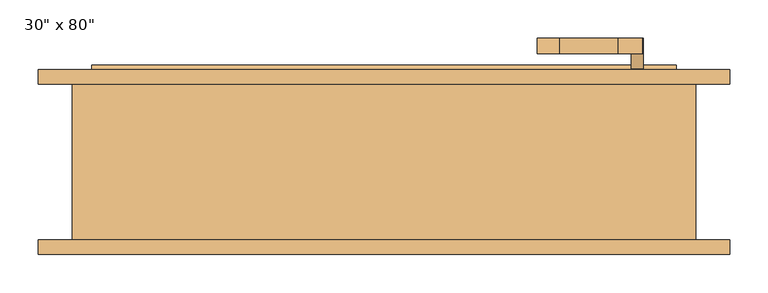
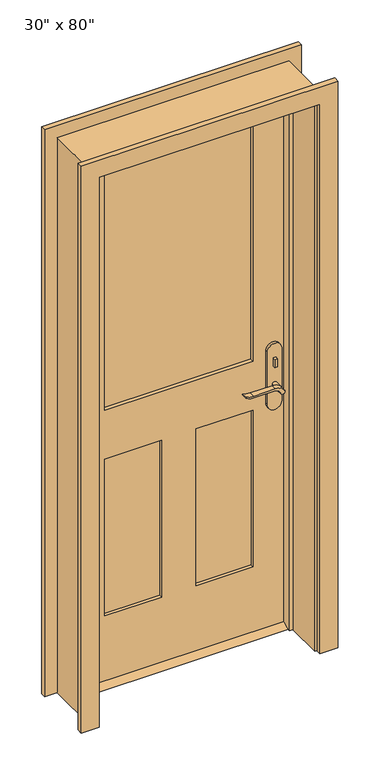
"""IFC4 building model written with IfcOpenShell, lengths in millimetres: door geometry."""

from ifc_helpers import new_model, si_unit, point, frame, frame_2d, origin, place, context, project, spatial, polyline, circle_curve, trimmed, segment, composite_curve, outline, extrude, faceted_brep, source, transform, mapped, element, save


def door_f50bbf81(model_context):
    return source(origin(), model_context, "Body", "SolidModel", [
        extrude(outline(polyline([(63.5, 12.7), (98.425, 12.7), (123.825, 0.0), (38.1, 0.0), (63.5, 12.7)])), frame((-381.0, 0.0, 0.0), z_axis=(1.0, 0.0, 0.0), x_axis=(0.0, 1.0, 0.0)), (0.0, 0.0, 1.0), 762.0),
        extrude(outline(polyline([(335.2, 43.5), (325.2, 43.5), (325.2, 53.5), (335.2, 53.5), (335.2, 43.5)])), frame((0.0, 0.0, 981.9), z_axis=(0.0, 0.0, 1.0), x_axis=(1.0, 0.0, 0.0)), (0.0, 0.0, 1.0), 30.0),
        extrude(outline(composite_curve([segment(trimmed(circle_curve(frame_2d((996.9, 330.2)), 8.0), [point((996.9, 322.2))], [point((996.9, 338.2))], False, "CARTESIAN"), True, "CONTINUOUS"), segment(trimmed(circle_curve(frame_2d((996.9, 330.2)), 8.0), [point((996.9, 338.2))], [point((996.9, 322.2))], False, "CARTESIAN"), True, "CONTINUOUS")], self_intersect=False)), frame((0.0, 108.425, 0.0), z_axis=(0.0, 1.0, 0.0), x_axis=(0.0, 0.0, 1.0)), (0.0, 0.0, 1.0), 10.0),
        extrude(outline(composite_curve([segment(trimmed(circle_curve(frame_2d((897.1555521, 306.5324871)), 37.2832219), [point((919.0523287, 336.7081363))], [point((934.4, 304.8325667))], False, "CARTESIAN"), True, "CONTINUOUS"), segment(polyline([(934.4, 304.8325667), (934.4, 228.5564091)]), True, "CONTINUOUS"), segment(trimmed(circle_curve(frame_2d((1017.6850638, 228.6227909)), 83.2850902), [point((934.4, 228.5564091))], [point((939.4, 200.2))], True, "CARTESIAN"), True, "CONTINUOUS"), segment(polyline([(939.4, 200.2), (936.6135558, 200.2)]), True, "CONTINUOUS"), segment(trimmed(circle_curve(frame_2d((986.6709207, 232.1396612)), 59.3791355), [point((936.6135558, 200.2))], [point((927.4, 228.5564091))], False, "CARTESIAN"), True, "CONTINUOUS"), segment(polyline([(927.4, 228.5564091), (927.4, 304.8138099)]), True, "CONTINUOUS"), segment(trimmed(circle_curve(frame_2d((909.2738613, 304.8138099)), 18.1261387), [point((927.4, 304.8138099))], [point((914.4, 322.2))], True, "CARTESIAN"), True, "CONTINUOUS"), segment(trimmed(circle_curve(frame_2d((914.4, 330.2)), 8.0), [point((914.4, 322.2))], [point((919.0523287, 336.7081363))], False, "CARTESIAN"), True, "CONTINUOUS")], self_intersect=False)), frame((0.0, 3.5, 0.0), z_axis=(0.0, 1.0, 0.0), x_axis=(0.0, 0.0, 1.0)), (0.0, 0.0, 1.0), 20.0),
        extrude(outline(composite_curve([segment(trimmed(circle_curve(frame_2d((914.4, 330.2)), 8.0), [point((914.3999903, 322.2))], [point((919.0523287, 336.7081363))], False, "CARTESIAN"), True, "CONTINUOUS"), segment(trimmed(circle_curve(frame_2d((897.1555521, 306.5324871)), 37.2832219), [point((919.0523287, 336.7081363))], [point((934.4, 304.8325667))], False, "CARTESIAN"), True, "CONTINUOUS"), segment(polyline([(934.4, 304.8325667), (934.4, 228.5564091)]), True, "CONTINUOUS"), segment(trimmed(circle_curve(frame_2d((1017.6850638, 228.6227909)), 83.2850902), [point((934.4, 228.5564091))], [point((939.4, 200.2))], True, "CARTESIAN"), True, "CONTINUOUS"), segment(polyline([(939.4, 200.2), (936.6135558, 200.2)]), True, "CONTINUOUS"), segment(trimmed(circle_curve(frame_2d((986.6709207, 232.1396612)), 59.3791355), [point((936.6135558, 200.2))], [point((927.4, 228.5564091))], False, "CARTESIAN"), True, "CONTINUOUS"), segment(polyline([(927.4, 228.5564091), (927.4, 304.8138122)]), True, "CONTINUOUS"), segment(trimmed(circle_curve(frame_2d((909.2738682, 304.8138122)), 18.1261318), [point((927.4, 304.8138122))], [point((914.3999903, 322.2))], True, "CARTESIAN"), True, "CONTINUOUS")], self_intersect=False)), frame((0.0, 138.425, 0.0), z_axis=(0.0, 1.0, 0.0), x_axis=(0.0, 0.0, 1.0)), (0.0, 0.0, 1.0), 20.0),
        extrude(outline(composite_curve([segment(trimmed(circle_curve(frame_2d((914.4, 330.2)), 8.0), [point((914.4, 322.2))], [point((914.4, 338.2))], False, "CARTESIAN"), True, "CONTINUOUS"), segment(trimmed(circle_curve(frame_2d((914.4, 330.2)), 8.0), [point((914.4, 338.2))], [point((914.4, 322.2))], False, "CARTESIAN"), True, "CONTINUOUS")], self_intersect=False)), frame((0.0, 23.5, 0.0), z_axis=(0.0, 1.0, 0.0), x_axis=(0.0, 0.0, 1.0)), (0.0, 0.0, 1.0), 30.0),
        extrude(outline(composite_curve([segment(trimmed(circle_curve(frame_2d((914.4, 330.2)), 8.0), [point((914.4, 322.2))], [point((914.4, 338.2))], False, "CARTESIAN"), True, "CONTINUOUS"), segment(trimmed(circle_curve(frame_2d((914.4, 330.2)), 8.0), [point((914.4, 338.2))], [point((914.4, 322.2))], False, "CARTESIAN"), True, "CONTINUOUS")], self_intersect=False)), frame((0.0, 108.425, 0.0), z_axis=(0.0, 1.0, 0.0), x_axis=(0.0, 0.0, 1.0)), (0.0, 0.0, 1.0), 30.0),
        extrude(outline(composite_curve([segment(polyline([(844.4, 355.2), (1039.4, 355.2)]), True, "CONTINUOUS"), segment(trimmed(circle_curve(frame_2d((1039.4, 330.2)), 25.0), [point((1039.4, 355.2))], [point((1039.4, 305.2))], False, "CARTESIAN"), True, "CONTINUOUS"), segment(polyline([(1039.4, 305.2), (844.4, 305.2)]), True, "CONTINUOUS"), segment(trimmed(circle_curve(frame_2d((844.4, 330.2)), 25.0), [point((844.4, 305.2))], [point((844.4, 355.2))], False, "CARTESIAN"), True, "CONTINUOUS")], self_intersect=False)), frame((0.0, 53.5, 0.0), z_axis=(0.0, 1.0, 0.0), x_axis=(0.0, 0.0, 1.0)), (0.0, 0.0, 1.0), 10.0),
        extrude(outline(composite_curve([segment(polyline([(844.4, 355.2), (1039.4, 355.2)]), True, "CONTINUOUS"), segment(trimmed(circle_curve(frame_2d((1039.4, 330.2)), 25.0), [point((1039.4, 355.2))], [point((1039.4, 305.2))], False, "CARTESIAN"), True, "CONTINUOUS"), segment(polyline([(1039.4, 305.2), (844.4, 305.2)]), True, "CONTINUOUS"), segment(trimmed(circle_curve(frame_2d((844.4, 330.2)), 25.0), [point((844.4, 305.2))], [point((844.4, 355.2))], False, "CARTESIAN"), True, "CONTINUOUS")], self_intersect=False)), frame((0.0, 98.425, 0.0), z_axis=(0.0, 1.0, 0.0), x_axis=(0.0, 0.0, 1.0)), (0.0, 0.0, 1.0), 10.0),
        extrude(outline(polyline([(2032.0, -381.0), (12.7, -381.0), (12.7, 381.0), (2032.0, 381.0), (2032.0, -381.0)]), holes=[polyline([(1016.0, -260.35), (1911.35, -260.35), (1911.35, 260.35), (1016.0, 260.35), (1016.0, -260.35)]), polyline([(835.025, -60.325), (254.0, -60.325), (254.0, -260.35), (835.025, -260.35), (835.025, -60.325)]), polyline([(835.025, 260.35), (254.0, 260.35), (254.0, 60.325), (835.025, 60.325), (835.025, 260.35)])]), frame((0.0, 63.5, 0.0), z_axis=(0.0, 1.0, 0.0), x_axis=(0.0, 0.0, 1.0)), (0.0, 0.0, 1.0), 34.925),
        faceted_brep([(406.4, 98.425, 0.0), (406.4, -104.775, 0.0), (381.0, -104.775, 0.0), (381.0, 28.575, 0.0), (368.3, 28.575, 0.0), (368.3, 63.5, 0.0), (381.0, 63.5, 0.0), (381.0, 98.425, 0.0), (406.4, 98.425, 2057.4), (406.4, -104.775, 2057.4), (-406.4, -104.775, 2057.4), (-406.4, -104.775, 0.0), (-381.0, -104.775, 0.0), (-381.0, -104.775, 2032.0), (381.0, -104.775, 2032.0), (381.0, 28.575, 2032.0), (-381.0, 28.575, 2032.0), (-381.0, 28.575, 0.0), (-368.3, 28.575, 0.0), (-368.3, 28.575, 2019.3), (368.3, 28.575, 2019.3), (368.3, 63.5, 2019.3), (-368.3, 63.5, 2019.3), (-368.3, 63.5, 0.0), (-381.0, 63.5, 0.0), (-381.0, 63.5, 2032.0), (381.0, 63.5, 2032.0), (381.0, 98.425, 2032.0), (-381.0, 98.425, 2032.0), (-381.0, 98.425, 0.0), (-406.4, 98.425, 0.0), (-406.4, 98.425, 2057.4)], [[[0, 1, 2, 3, 4, 5, 6, 7]], [[1, 0, 8, 9]], [[2, 1, 9, 10, 11, 12, 13, 14]], [[3, 2, 14, 15]], [[4, 3, 15, 16, 17, 18, 19, 20]], [[5, 4, 20, 21]], [[6, 5, 21, 22, 23, 24, 25, 26]], [[7, 6, 26, 27]], [[0, 7, 27, 28, 29, 30, 31, 8]], [[9, 8, 31, 10]], [[15, 14, 13, 16]], [[21, 20, 19, 22]], [[27, 26, 25, 28]], [[30, 29, 24, 23, 18, 17, 12, 11]], [[10, 31, 30, 11]], [[16, 13, 12, 17]], [[22, 19, 18, 23]], [[28, 25, 24, 29]]]),
        extrude(outline(polyline([(-60.325, 75.1416667), (-260.35, 75.1416667), (-260.35, 86.7833333), (-60.325, 86.7833333), (-60.325, 75.1416667)])), frame((0.0, 0.0, 254.0), z_axis=(0.0, 0.0, 1.0), x_axis=(1.0, 0.0, 0.0)), (0.0, 0.0, 1.0), 581.025),
        extrude(outline(polyline([(260.35, 75.1416667), (60.325, 75.1416667), (60.325, 86.7833333), (260.35, 86.7833333), (260.35, 75.1416667)])), frame((0.0, 0.0, 254.0), z_axis=(0.0, 0.0, 1.0), x_axis=(1.0, 0.0, 0.0)), (0.0, 0.0, 1.0), 581.025),
        extrude(outline(polyline([(260.35, 77.47), (-260.35, 77.47), (-260.35, 84.455), (260.35, 84.455), (260.35, 77.47)])), frame((0.0, 0.0, 1016.0), z_axis=(0.0, 0.0, 1.0), x_axis=(1.0, 0.0, 0.0)), (0.0, 0.0, 1.0), 895.35),
        extrude(outline(polyline([(0.0, -450.85), (0.0, -387.35), (2038.35, -387.35), (2038.35, 387.35), (0.0, 387.35), (0.0, 450.85), (2101.85, 450.85), (2101.85, -450.85), (0.0, -450.85)])), frame((0.0, -123.825, 0.0), z_axis=(0.0, 1.0, 0.0), x_axis=(0.0, 0.0, 1.0)), (0.0, 0.0, 1.0), 19.05),
        extrude(outline(polyline([(0.0, -450.85), (0.0, -387.35), (2038.35, -387.35), (2038.35, 387.35), (0.0, 387.35), (0.0, 450.85), (2101.85, 450.85), (2101.85, -450.85), (0.0, -450.85)])), frame((0.0, 98.425, 0.0), z_axis=(0.0, 1.0, 0.0), x_axis=(0.0, 0.0, 1.0)), (0.0, 0.0, 1.0), 19.05),
    ])


if __name__ == "__main__":
    model = new_model("IFC4")
    model_context = context("Model", 3, world=origin())
    ifc_project = project(units=[si_unit("LENGTHUNIT", "METRE", prefix="MILLI")], contexts=[model_context])
    site = spatial("IfcSite", under=ifc_project)
    building = spatial("IfcBuilding", under=site)
    placement = place(None, origin())
    door_shape = door_f50bbf81(model_context)
    element("IfcDoor", 1, ObjectType="30\" x 80\"", at=placement, inside=building, context=model_context, shape_type="MappedRepresentation", body=[
        mapped(door_shape, transform((0.0, 0.0, 0.0), x_axis=(1.0, 0.0, 0.0), y_axis=(0.0, 1.0, 0.0), z_axis=(0.0, 0.0, 1.0))),
    ])
    save(model, "model.ifc")

# Revit data of these elements
# Type "30\" x 80\""
#   Type Mark = "8"
#   Assembly Code = "B2030100"
#   Analytic Construction = "French door, wood frame with single glass"
#   Top Rail = 0' - 4 3/4"
#   Threshold Offset [instance default] = 0' - 0 1/2"
#   Thickness = 0' - 1 3/8"
#   Thermal Resistance (R) = 1.0696 (h·ft²·°F)/BTU
#   Swing Angle [instance default] = 90.00°
#   Stiles = 0' - 4 3/4"
#   Rough Width = 2' - 8"
#   Rough Height = 6' - 9"
#   Lock Rail = 0' - 7 1/8"
#   Height = 6' - 8"
#   Width = 2' - 6"
#   Heat Transfer Coefficient (U) = 0.9350 BTU/(h·ft²·°F)
#   Door Offset [instance default] = 0' - 0"
#   Bottom Rail = 0' - 9 1/2"
#   Threshold [instance default] = yes
#   Function = 1
#   Exterior Trim [instance default] = yes
#   Trim Material = Cherry
#   Threshold Material = Cherry
#   Panel Material = Cherry
#   Glazing = Glass
#   Frame Material = Cherry
#   Door Handle Material = Aluminum
#   Visual Light Transmittance = 0
#   Solar Heat Gain Coefficient = 0
#   Wall Closure = (empty or 0)
#   Construction Type = (empty or 0)
# Element 1 (IfcDoor, "30\" x 80\"")
#   Materials on its faces: "Cherry", "Aluminum", "Glass"
# Materials
#   "Cherry": class "Wood", colour RGB 226 177 128, transparency 0, Description = "Prunus Serotina", Cost = 0
#   "Glass": class "Glass", colour RGB 0 128 192, transparency 0.75, Description = "Soda Lime Glass", Cost = 0
#   "Aluminum": class "Metal", colour RGB 247 247 247, transparency 0, Description = "Aluminum 6061", Cost = 0
